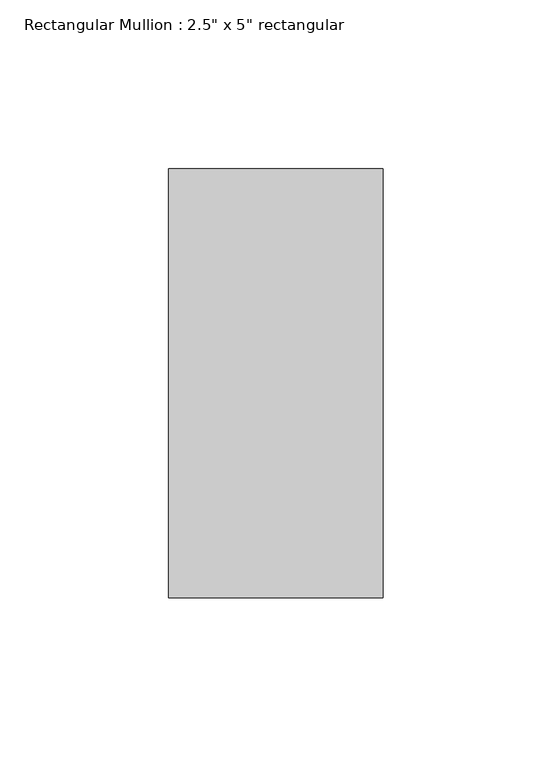
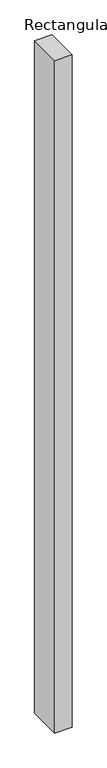
"""IFC4 building model written with IfcOpenShell, lengths in millimetres: member geometry."""

from ifc_helpers import new_model, si_unit, frame, origin, place, context, project, spatial, polyline, outline, extrude, source, transform, mapped, element, save


def member_cf032248(model_context):
    return source(origin(), model_context, "Body", "SweptSolid", [
        extrude(outline(polyline([(0.0, 63.5), (0.0, -63.5), (-63.5, -63.5), (-63.5, 63.5), (0.0, 63.5)])), frame((0.0, 0.0, -2598.8380434), z_axis=(0.0, 0.0, 1.0), x_axis=(1.0, 0.0, 0.0)), (0.0, 0.0, 1.0), 2598.8380434),
    ])


if __name__ == "__main__":
    model = new_model("IFC4")
    model_context = context("Model", 3, world=origin())
    ifc_project = project(units=[si_unit("LENGTHUNIT", "METRE", prefix="MILLI")], contexts=[model_context])
    site = spatial("IfcSite", under=ifc_project)
    building = spatial("IfcBuilding", under=site)
    placement = place(None, origin())
    member_shape = member_cf032248(model_context)
    element("IfcMember", 1, ObjectType="Rectangular Mullion : 2.5\" x 5\" rectangular", at=placement, inside=building, context=model_context, shape_type="MappedRepresentation", body=[
        mapped(member_shape, transform((0.0, 0.0, 0.0), x_axis=(1.0, 0.0, 0.0), y_axis=(0.0, 1.0, 0.0), z_axis=(0.0, 0.0, 1.0))),
    ])
    save(model, "model.ifc")

# Revit data of these elements
# Type "Rectangular Mullion : 2.5\" x 5\" rectangular"
#   built-in parameter 1007304 = 0.416667 (stored number, unit not read)
#   built-in parameter 1007301 = 0.104167 (stored number, unit not read)
#   built-in parameter 1007300 = 0.104167 (stored number, unit not read)
# Element 1 (IfcMember, "Rectangular Mullion : 2.5\" x 5\" rectangular")
#   Materials on its faces: "Aluminum"
# Materials
#   "Aluminum": class "Metal", colour RGB 247 247 247, transparency 0, Description = "Aluminum 6061", Cost = 0
